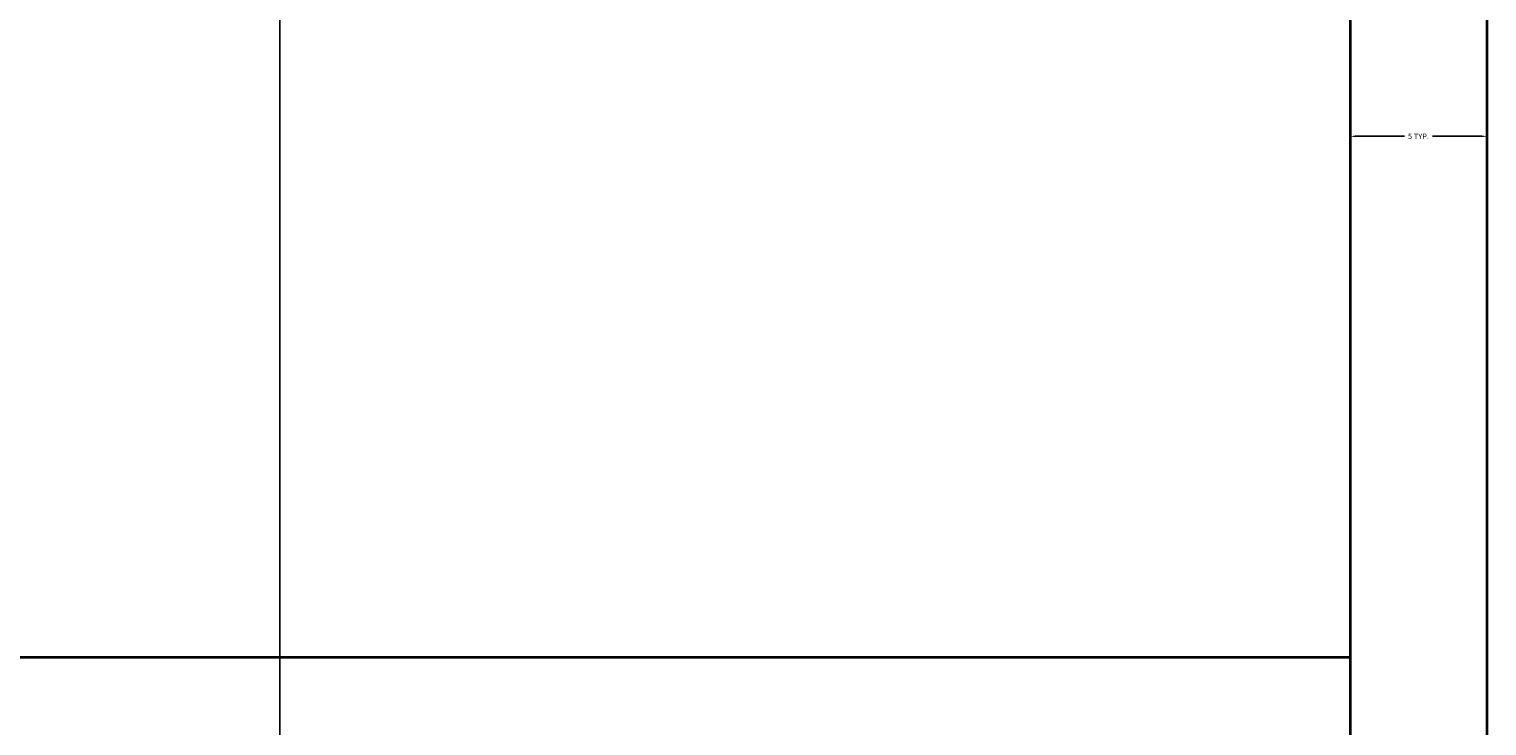
# Model space of a CAD drawing. Units: inches. Extents: x 1088 to 1703, y 668 to 1875.
# Tile 35 of 45: x 1542 to 1590, y 1606 to 1629. Entities that reach past the tile are written whole.
import ezdxf

# ---------------------------------------------------------------- set-up
doc = ezdxf.new("R2010")
doc.units = ezdxf.units.IN
doc.layers.add('A-ANNO-DIMS', color=2, linetype='Continuous', lineweight=18)
doc.layers.add('A-WALL', color=7, linetype='Continuous', lineweight=35)
doc.styles.get("Standard").update_dxf_attribs({"font": 'arial.ttf'})
doc.dimstyles.get("Standard").update_dxf_attribs({"dimtxt": 0.18, "dimasz": 0.18, "dimexe": 0.18, "dimexo": 0.0625, "dimgap": 0.09, "dimtad": 0, "dimtih": 1, "dimtoh": 1, "dimdec": 4, "dimzin": 0, "dimdsep": 46, "dimtxsty": 'Standard', "dimcen": 0.09, "dimadec": 0, "dimazin": 0, "dimtfac": 1, "dimtdec": 4, "dimtofl": 0, "dimtmove": 0, "dimatfit": 3, "dimfxl": 1, "dimtolj": 1, "dimtzin": 0, "dimarcsym": 0})

# ---------------------------------------------------------------- blocks, each defined once
blk = doc.blocks.new('*D21')
at = {"layer": 'A-ANNO-DIMS', "color": 0, "lineweight": -2, "transparency": 16777216}
for p, q in [((1585.845, 1629.254), (1585.845, 1625.537)), ((1590.345, 1629.254), (1590.345, 1625.537)), ((1586.025, 1625.717), (1587.637, 1625.717)), ((1590.165, 1625.717), (1588.553, 1625.717))]:
    blk.add_line(p, q, dxfattribs=at)
at = {"layer": 'A-ANNO-DIMS', "color": 0, "transparency": 16777216}
for points in [[(1586.025, 1625.747), (1586.025, 1625.687), (1585.845, 1625.717)], [(1590.165, 1625.747), (1590.165, 1625.687), (1590.345, 1625.717)]]:
    blk.add_solid(points, dxfattribs=at)
at = {"layer": 'Defpoints', "color": 0, "transparency": 16777216}
for p in [(1585.845, 1629.317), (1590.345, 1629.317), (1590.345, 1625.717)]:
    blk.add_point(p, dxfattribs=at)
at = {"layer": 'A-ANNO-DIMS', "color": 0, "transparency": 16777216, "insert": (1588.095, 1625.717), "char_height": 0.18, "attachment_point": 5}
blk.add_mtext('\\A1;5 TYP.', dxfattribs=at)
blk = doc.blocks.new('*D32')
at = {"layer": 'A-ANNO-DIMS', "color": 0, "lineweight": -2, "transparency": 16777216}
for p, q in [((1550.595, 1373.121), (1550.595, 1857.788)), ((1585.845, 1360.983), (1585.845, 1857.788)), ((1550.775, 1857.608), (1567.825, 1857.608)), ((1585.665, 1857.608), (1568.614, 1857.608))]:
    blk.add_line(p, q, dxfattribs=at)
at = {"layer": 'A-ANNO-DIMS', "color": 0, "transparency": 16777216}
for points in [[(1550.775, 1857.638), (1550.775, 1857.578), (1550.595, 1857.608)], [(1585.665, 1857.638), (1585.665, 1857.578), (1585.845, 1857.608)]]:
    blk.add_solid(points, dxfattribs=at)
at = {"layer": 'Defpoints', "color": 0, "transparency": 16777216}
for p in [(1585.845, 1857.608), (1550.595, 1373.058), (1585.845, 1360.921)]:
    blk.add_point(p, dxfattribs=at)
at = {"layer": 'A-ANNO-DIMS', "color": 0, "transparency": 16777216, "insert": (1568.22, 1857.608), "char_height": 0.18, "attachment_point": 5}
blk.add_mtext('\\A1;35.25', dxfattribs=at)

msp = doc.modelspace()

# ---------------------------------------------------------------- linework, layer by layer
at = {"layer": 'A-WALL'}
for p, q in [((1590.345, 1673.058), (1590.345, 1539.558)), ((1585.845, 1668.558), (1585.845, 1544.058)), ((1585.845, 1668.558), (1585.845, 1608.558)), ((1585.845, 1608.558), (1489.845, 1608.558))]:
    msp.add_line(p, q, dxfattribs=at)

# ---------------------------------------------------------------- dimensions: what is measured, and where the dimension line sits
at = {"layer": 'A-ANNO-DIMS'}
dim = msp.add_linear_dim(base=(1585.845, 1857.608), p1=(1550.595, 1373.058), p2=(1585.845, 1360.921), dimstyle='Standard', override={"dimdec": 2, "dimlfac": 1, "dimrnd": 0, "dimzin": 0, "dimdsep": 46, "dimlunit": 2}, dxfattribs=at)
dim.commit()
dim.dimension.update_dxf_attribs({"geometry": '*D32', "text_midpoint": (1568.22, 1857.608)})
dim = msp.add_linear_dim(base=(1590.344800082, 1625.716851167), p1=(1585.844800082, 1629.316851167), p2=(1590.344800082, 1629.316851167), text='<> TYP.', dimstyle='Standard', override={"dimdec": 0, "dimlfac": 1, "dimrnd": 0, "dimzin": 0, "dimdsep": 46, "dimlunit": 2}, dxfattribs=at)
dim.commit()
dim.dimension.update_dxf_attribs({"geometry": '*D21', "text_midpoint": (1588.094800082, 1625.716851167)})

doc.saveas('drawing.dxf')
